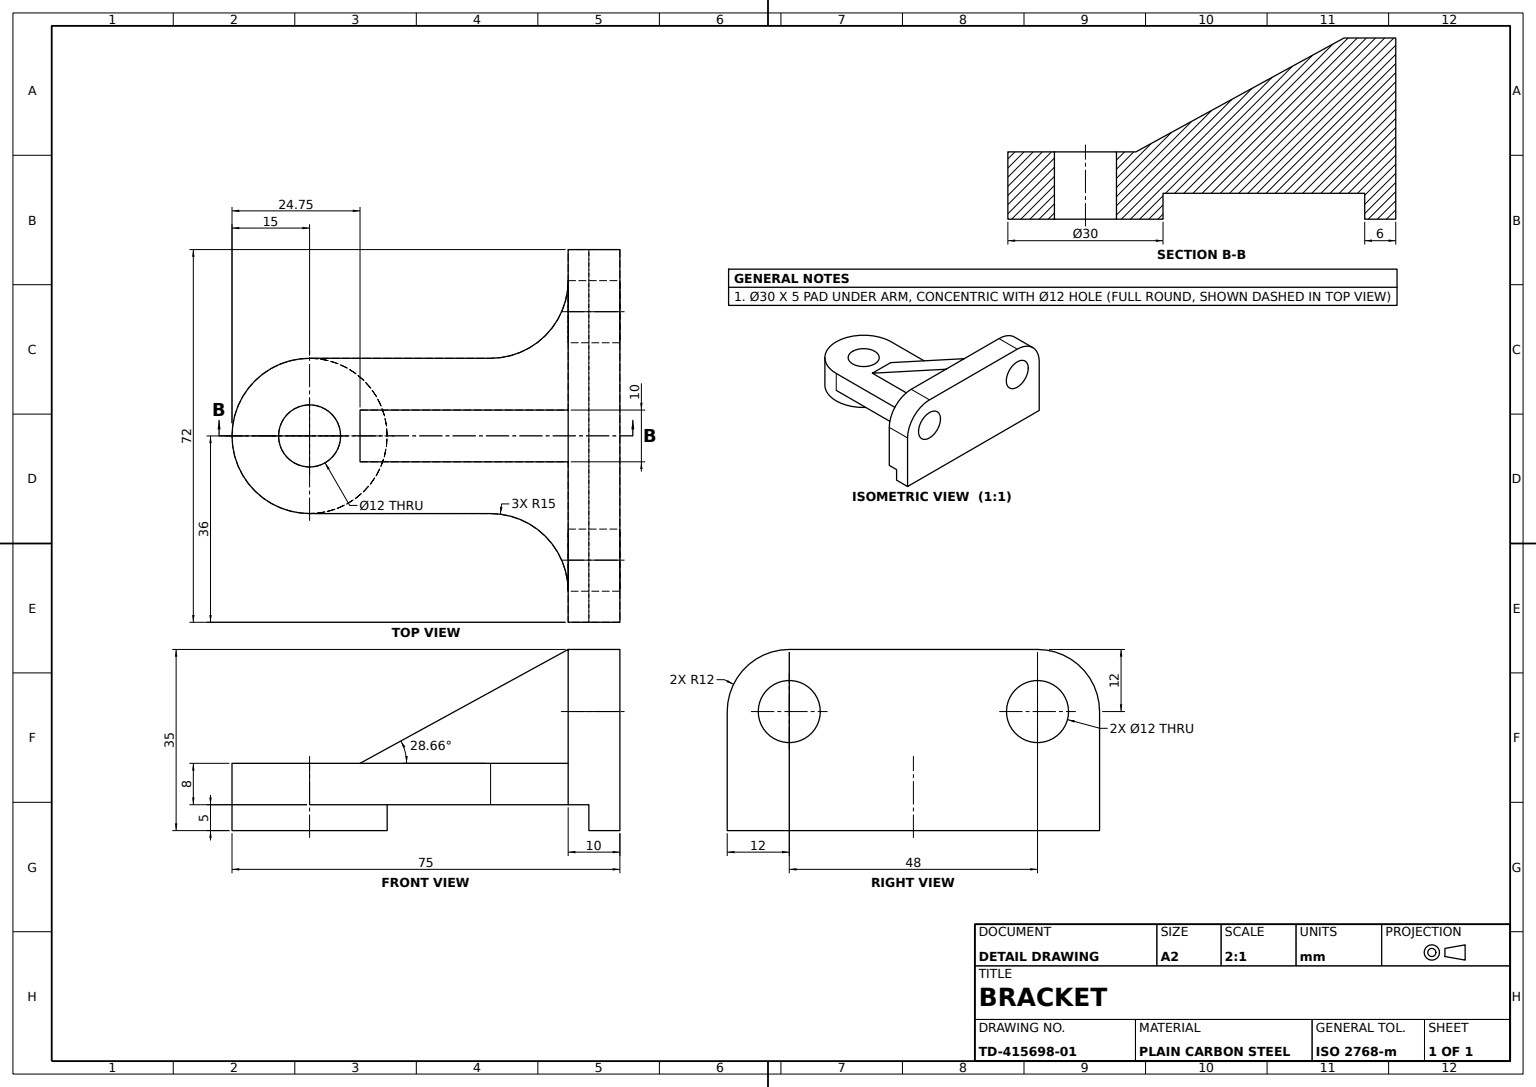
from build123d import *

# Parameters (mm, degrees)
MOUNTING_PLATE_DEPTH     = 10
PLATE_NOTCH_SKETCH_W     = 4
PLATE_NOTCH_SKETCH_H     = 5
PLATE_NOTCH_CUT_DEPTH    = 72
PIVOT_ARM_DEPTH          = 8
PIVOT_START              = 5
PIVOT_BOSS_SKETCH_R      = 15
PIVOT_BOSS_30_DEPTH      = 5
PLATE_HOLES_SKETCH_R     = 6
PLATE_HOLES_2X_12_DEPTH  = 10
PIVOT_HOLE_SKETCH_R      = 6
PIVOT_HOLE_12_DEPTH      = 13
GUSSET_BLANK_DEPTH       = 42
GUSSET_TAPER_CUT_DEPTH   = 30
GUSSET_EDGE_TRIM_A_DEPTH = 1
GUSSET_EDGE_TRIM_B_DEPTH = 1


with BuildPart() as part:
    # Plate Profile Sketch → Mounting Plate (new body)
    with BuildSketch(Plane.XY):
        with BuildLine():
            Line((0, 0), (0, -23))
            Line((0, -23), (72, -23))
            Line((72, -23), (72, 0))
            ThreePointArc((72, 0), (68.485281374, 8.485281374), (60, 12))
            Line((60, 12), (12, 12))
            ThreePointArc((12, 12), (3.514718626, 8.485281374), (0, 0))
        make_face()
    extrude(amount=MOUNTING_PLATE_DEPTH)

    # Plate Notch Sketch → Plate Notch Cut (cut)
    with BuildSketch(Plane.ZY):
        with Locations((8, -20.5)):
            Rectangle(PLATE_NOTCH_SKETCH_W, PLATE_NOTCH_SKETCH_H)
    extrude(amount=-PLATE_NOTCH_CUT_DEPTH, mode=Mode.SUBTRACT)

    # Arm Profile Sketch → Pivot Arm (add)
    with BuildSketch(Plane.XZ.offset(18)):
        with BuildLine():
            Line((6, 10), (66, 10))
            ThreePointArc((66, 10), (55.393398282, 14.393398282), (51, 25))
            Line((51, 25), (51, 60))
            ThreePointArc((51, 60), (36, 75), (21, 60))
            Line((21, 60), (21, 25))
            ThreePointArc((21, 25), (16.606601718, 14.393398282), (6, 10))
        make_face()
    extrude(amount=-PIVOT_ARM_DEPTH)

    # Pivot Boss Sketch → Pivot Boss Ø30 (add)
    with BuildSketch(Plane.XZ.offset(18).offset(PIVOT_START)):
        with Locations(Location((36, 60, 0), (0, 0, 270))):
            Circle(PIVOT_BOSS_SKETCH_R)
    extrude(amount=-PIVOT_BOSS_30_DEPTH)

    # Plate Holes Sketch → Plate Holes 2xØ12 (cut)
    with BuildSketch(Plane.XY.offset(10)):
        with Locations((12, 0)):
            Circle(PLATE_HOLES_SKETCH_R)
        with Locations((60, 0)):
            Circle(PLATE_HOLES_SKETCH_R)
    extrude(amount=-PLATE_HOLES_2X_12_DEPTH, mode=Mode.SUBTRACT)

    # Pivot Hole Sketch → Pivot Hole Ø12 (cut)
    with BuildSketch(Plane.XZ.offset(23)):
        with Locations(Location((36, 60, 0), (0, 0, 270))):
            Circle(PIVOT_HOLE_SKETCH_R)
    extrude(amount=-PIVOT_HOLE_12_DEPTH, mode=Mode.SUBTRACT)

    # Gusset Profile Sketch → Gusset Blank (add)
    with BuildSketch(Plane.ZY):
        Polygon((10, -10), (50.245930421, -10), (10, 12), align=None)
    extrude(amount=-GUSSET_BLANK_DEPTH)

    # Gusset Taper Sketch → Gusset Taper Cut (cut)
    with BuildSketch(Plane.ZY):
        Polygon((10, 12), (10, -10), (50.245930421, -10), align=None)
    extrude(amount=-GUSSET_TAPER_CUT_DEPTH, mode=Mode.SUBTRACT)

    # Gusset Edge Trim A Sketch → Gusset Edge Trim A (cut)
    with BuildSketch(Plane.ZY.offset(-30)):
        Polygon((10, 12), (10, -10), (50.245930421, -10), align=None)
    extrude(amount=-GUSSET_EDGE_TRIM_A_DEPTH, mode=Mode.SUBTRACT)

    # Gusset Edge Trim B Sketch → Gusset Edge Trim B (cut)
    with BuildSketch(Plane(origin=(42, 0, 0), x_dir=(0, 0, -1), z_dir=(1, 0, 0))):
        Polygon((-50.245930421, -10), (-10, -10), (-10, 12), align=None)
    extrude(amount=-GUSSET_EDGE_TRIM_B_DEPTH, mode=Mode.SUBTRACT)


solid = part.part
